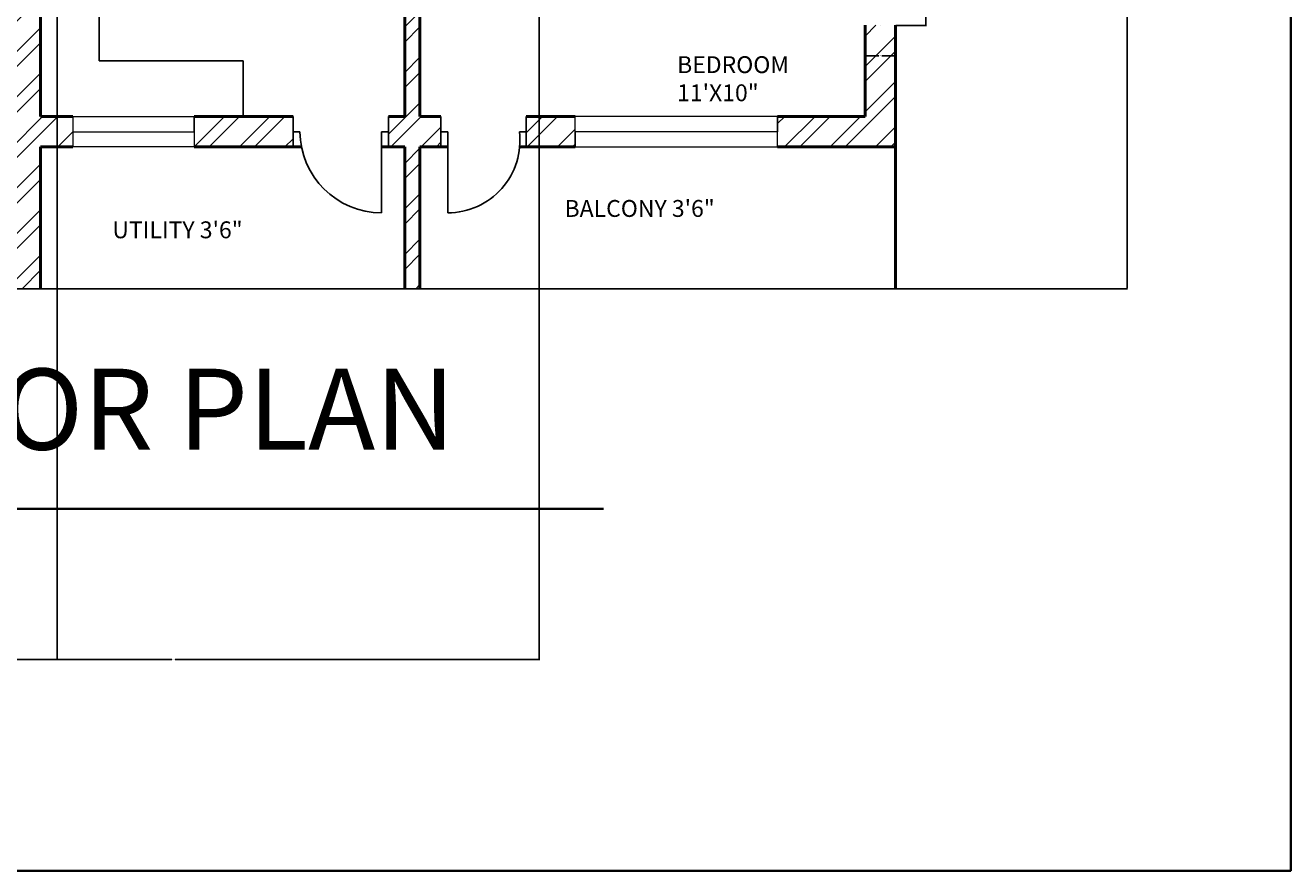
# Model space of a CAD drawing. Units: inches. Extents: x 1980 to 2738, y 1471 to 2568.
# Tile 11 of 22: x 2363 to 2738, y 1471 to 1722. Entities that reach past the tile are written whole.
import ezdxf

# ---------------------------------------------------------------- set-up
doc = ezdxf.new("R2010")
doc.units = ezdxf.units.IN
for name, color, linetype, lineweight in [('A-ANNO-DIMS', 2, 'Continuous', 18), ('A-ANNO-TTLB', 7, 'Continuous', 35), ('A-AREA-IDEN', 7, 'Continuous', 18), ('A-DOOR', 31, 'Continuous', 25), ('A-FLOR-BALC', 7, 'Continuous', 25), ('A-FLOR-CASE', 8, 'Continuous', 25), ('A-GLAZ', 141, 'Continuous', 18), ('A-WALL', 7, 'Continuous', 50)]:
    doc.layers.add(name, color=color, linetype=linetype, lineweight=lineweight)
doc.layers.add('A-WALL-PATT', color=9, linetype='Continuous', lineweight=13, true_color=0xd19cc7)
doc.styles.get("Standard").update_dxf_attribs({"font": 'arial.ttf'})
doc.dimstyles.get("Standard").update_dxf_attribs({"dimtxt": 0.18, "dimasz": 0.18, "dimexe": 0.18, "dimexo": 0.0625, "dimgap": 0.09, "dimtad": 0, "dimtih": 1, "dimtoh": 1, "dimdec": 4, "dimzin": 0, "dimdsep": 46, "dimtxsty": 'Standard', "dimcen": 0.09, "dimadec": 0, "dimazin": 0, "dimtfac": 1, "dimtdec": 4, "dimtofl": 0, "dimtmove": 0, "dimatfit": 3, "dimfxl": 1, "dimtolj": 1, "dimtzin": 0, "dimarcsym": 0})

# ---------------------------------------------------------------- blocks, each defined once
blk = doc.blocks.new('WIN-60IN-WALL')
for p, q in [((0, 9), (0, 0)), ((60, 9), (0, 9)), ((60, 4.5), (60, 9)), ((60, 9), (60, 0)), ((0, 0), (0, 4.5)), ((0, 4.5), (60, 4.5)), ((0, 0), (60, 0))]:
    blk.add_line(p, q)
blk = doc.blocks.new('*D29')
at = {"layer": 'A-ANNO-DIMS', "color": 0, "lineweight": -2, "transparency": 16777216}
for p, q in [((2621.15, 1781.73), (2630.26, 1781.73)), ((2630.08, 1781.55), (2630.08, 1751.92)), ((2630.08, 1721.91), (2630.08, 1751.55)), ((2621.15, 1721.73), (2630.26, 1721.73))]:
    blk.add_line(p, q, dxfattribs=at)
at = {"layer": 'A-ANNO-DIMS', "color": 0, "transparency": 16777216}
for points in [[(2630.05, 1781.55), (2630.11, 1781.55), (2630.08, 1781.73)], [(2630.05, 1721.91), (2630.11, 1721.91), (2630.08, 1721.73)]]:
    blk.add_solid(points, dxfattribs=at)
at = {"layer": 'Defpoints', "color": 0, "transparency": 16777216}
for p in [(2621.08, 1781.73), (2630.08, 1781.73), (2621.08, 1721.73)]:
    blk.add_point(p, dxfattribs=at)
at = {"layer": 'A-ANNO-DIMS', "color": 0, "transparency": 16777216, "insert": (2630.08, 1751.73), "char_height": 0.18, "attachment_point": 5}
blk.add_mtext('\\A1;WINDOW 60 TYP.', dxfattribs=at)
blk = doc.blocks.new('*D30')
at = {"layer": 'A-ANNO-DIMS', "color": 0, "lineweight": -2, "transparency": 16777216}
for p, q in [((2612.08, 1721.67), (2612.08, 1712.55)), ((2621.08, 1721.67), (2621.08, 1712.55)), ((2612.26, 1712.73), (2616.13, 1712.73)), ((2620.9, 1712.73), (2617.04, 1712.73))]:
    blk.add_line(p, q, dxfattribs=at)
at = {"layer": 'A-ANNO-DIMS', "color": 0, "transparency": 16777216}
for points in [[(2612.26, 1712.76), (2612.26, 1712.7), (2612.08, 1712.73)], [(2620.9, 1712.76), (2620.9, 1712.7), (2621.08, 1712.73)]]:
    blk.add_solid(points, dxfattribs=at)
at = {"layer": 'Defpoints', "color": 0, "transparency": 16777216}
for p in [(2612.08, 1721.73), (2621.08, 1721.73), (2621.08, 1712.73)]:
    blk.add_point(p, dxfattribs=at)
at = {"layer": 'A-ANNO-DIMS', "color": 0, "transparency": 16777216, "insert": (2616.58, 1712.73), "char_height": 0.18, "attachment_point": 5}
blk.add_mtext('\\A1;9 TYP.', dxfattribs=at)
blk = doc.blocks.new('*D37')
at = {"layer": 'A-ANNO-DIMS', "color": 0, "lineweight": -2, "transparency": 16777216}
for p, q in [((2579.97, 2011.21), (2689.91, 2011.21)), ((2689.73, 2011.03), (2689.73, 1827.64)), ((2689.73, 1643.89), (2689.73, 1827.27)), ((2621.15, 1643.71), (2689.91, 1643.71))]:
    blk.add_line(p, q, dxfattribs=at)
at = {"layer": 'A-ANNO-DIMS', "color": 0, "transparency": 16777216}
for points in [[(2689.7, 2011.03), (2689.76, 2011.03), (2689.73, 2011.21)], [(2689.7, 1643.89), (2689.76, 1643.89), (2689.73, 1643.71)]]:
    blk.add_solid(points, dxfattribs=at)
at = {"layer": 'Defpoints', "color": 0, "transparency": 16777216}
for p in [(2579.9, 2011.21), (2689.73, 2011.21), (2621.08, 1643.71)]:
    blk.add_point(p, dxfattribs=at)
at = {"layer": 'A-ANNO-DIMS', "color": 0, "transparency": 16777216, "insert": (2689.73, 1827.46), "char_height": 0.18, "attachment_point": 5}
blk.add_mtext('\\A1;367.5', dxfattribs=at)
blk = doc.blocks.new('*D41')
at = {"layer": 'A-ANNO-DIMS', "color": 0, "lineweight": -2, "transparency": 16777216}
for p, q in [((2298.65, 2095.14), (2298.65, 1533.71)), ((2515.4, 2095.14), (2515.4, 1533.71)), ((2298.83, 1533.89), (2406.56, 1533.89)), ((2515.22, 1533.89), (2407.49, 1533.89))]:
    blk.add_line(p, q, dxfattribs=at)
at = {"layer": 'A-ANNO-DIMS', "color": 0, "transparency": 16777216}
for points in [[(2298.83, 1533.92), (2298.83, 1533.86), (2298.65, 1533.89)], [(2515.22, 1533.92), (2515.22, 1533.86), (2515.4, 1533.89)]]:
    blk.add_solid(points, dxfattribs=at)
at = {"layer": 'Defpoints', "color": 0, "transparency": 16777216}
for p in [(2298.65, 2095.21), (2515.4, 2095.21), (2515.4, 1533.89)]:
    blk.add_point(p, dxfattribs=at)
at = {"layer": 'A-ANNO-DIMS', "color": 0, "transparency": 16777216, "insert": (2407.03, 1533.89), "char_height": 0.18, "attachment_point": 5}
blk.add_mtext('\\A1;216.75', dxfattribs=at)
blk = doc.blocks.new('*D57')
at = {"layer": 'A-ANNO-DIMS', "color": 0, "lineweight": -2, "transparency": 16777216}
for p, q in [((2351.81, 1792.14), (2351.81, 1533.71)), ((2372.53, 1792.14), (2372.53, 1533.71)), ((2351.99, 1533.89), (2361.77, 1533.89)), ((2372.35, 1533.89), (2362.56, 1533.89))]:
    blk.add_line(p, q, dxfattribs=at)
at = {"layer": 'A-ANNO-DIMS', "color": 0, "transparency": 16777216}
for points in [[(2351.99, 1533.92), (2351.99, 1533.86), (2351.81, 1533.89)], [(2372.35, 1533.92), (2372.35, 1533.86), (2372.53, 1533.89)]]:
    blk.add_solid(points, dxfattribs=at)
at = {"layer": 'Defpoints', "color": 0, "transparency": 16777216}
for p in [(2351.81, 1792.21), (2372.53, 1792.21), (2372.53, 1533.89)]:
    blk.add_point(p, dxfattribs=at)
at = {"layer": 'A-ANNO-DIMS', "color": 0, "transparency": 16777216, "insert": (2362.17, 1533.89), "char_height": 0.18, "attachment_point": 5}
blk.add_mtext('\\A1;20.72', dxfattribs=at)

msp = doc.modelspace()

# ---------------------------------------------------------------- hatches: boundary and pattern name
at = {"layer": 'A-WALL-PATT'}
h = msp.add_hatch(dxfattribs=at)
h.set_pattern_fill('ANSI32', color=256)
h.paths.add_polyline_path([(2257.5661, 2416.2064), (2257.5661, 2420.7064), (2250.5833, 2420.7064), (2250.5833, 2462.7064), (2246.0833, 2462.7064), (2246.0833, 2420.7064), (2237.0791, 2420.7064), (2237.0791, 2411.7064), (2246.0833, 2411.7064), (2246.0833, 2291.7064), (2242.6109, 2291.7064), (2242.6109, 2287.2064), (2246.0833, 2287.2064), (2250.5833, 2287.2064), (2250.5833, 2291.7064), (2250.5833, 2411.7064), (2257.5661, 2411.7064)])
h.paths.add_polyline_path([(2387.0396, 2416.2064), (2387.0396, 2420.7064), (2367.5833, 2420.7064), (2367.5833, 2462.7064), (2358.5833, 2462.7064), (2358.5833, 2420.7064), (2329.3087, 2420.7064), (2329.3087, 2411.7064), (2358.5833, 2411.7064), (2358.5833, 2321.7275), (2358.5833, 2309.7064), (2347.3089, 2309.7064), (2293.3089, 2309.7064), (2293.3089, 2259.0771), (2297.8089, 2259.0771), (2297.8089, 2305.2064), (2347.3089, 2305.2064), (2347.3089, 2284.7412), (2351.8089, 2284.7412), (2351.8089, 2305.2064), (2372.3188, 2305.2064), (2372.3761, 2284.3899), (2377.0295, 2284.3899), (2377.0295, 2299.3058), (2377.0295, 2305.2064), (2426.5295, 2305.2064), (2426.5295, 2257.5573), (2431.0295, 2257.5573), (2431.0295, 2309.7064), (2377.0295, 2309.7064), (2367.5833, 2309.7064), (2367.5833, 2321.7275), (2367.5833, 2411.7064), (2387.0396, 2411.7064)])
h.paths.add_polyline_path([(2448.5267, 2416.2064), (2448.5267, 2420.7064), (2423.0396, 2420.7064), (2423.0396, 2411.7064), (2448.5267, 2411.7064)])
h.paths.add_polyline_path([(2130.9128, 2416.2064), (2130.9128, 2420.7064), (2105.0833, 2420.7064), (2105.0833, 2386.6942), (2114.0833, 2386.6942), (2114.0833, 2411.7064), (2130.9128, 2411.7064)])
h.paths.add_polyline_path([(2212.9478, 2420.7064), (2190.9128, 2420.7064), (2190.9128, 2411.7064), (2212.9478, 2411.7064), (2212.9478, 2416.2064)])
h.paths.add_polyline_path([(2114.0833, 2326.6942), (2105.0833, 2326.6942), (2105.0833, 2291.7064), (2081.0833, 2291.7064), (2081.0833, 2287.2064), (2105.0833, 2287.2064), (2105.0833, 2276.1935), (2114.0833, 2276.1935), (2114.0833, 2287.2064), (2166.3825, 2287.2064), (2166.3825, 2289.4564), (2166.3825, 2291.7064), (2114.0833, 2291.7064)])
h.paths.add_polyline_path([(2114.0833, 2252.1935), (2105.0833, 2252.1935), (2105.0833, 2233.2064), (2081.0833, 2233.2064), (2081.0833, 2228.7064), (2105.0833, 2228.7064), (2105.0833, 2213.4478), (2114.0833, 2213.4478), (2114.0833, 2228.7064), (2195.0833, 2228.7064), (2199.5833, 2228.7064), (2208.4455, 2228.7064), (2208.4455, 2230.9564), (2208.4455, 2233.2064), (2199.5833, 2233.2064), (2199.5833, 2287.2064), (2206.8904, 2287.2064), (2206.8904, 2289.4564), (2206.8904, 2291.7064), (2189.446, 2291.7064), (2189.446, 2289.4564), (2189.446, 2287.2064), (2195.0833, 2287.2064), (2195.0833, 2233.2064), (2114.0833, 2233.2064)])
h.paths.add_polyline_path([(2114.0833, 2153.4478), (2109.5833, 2153.4478), (2105.0833, 2153.4478), (2105.0833, 2135.2374), (2114.0833, 2135.2374)], flags=17)
h.paths.add_polyline_path([(2135.9619, 2095.4081), (2140.1805, 2095.4081), (2140.1805, 2104.2064), (2114.0833, 2104.2064), (2114.0833, 2110.3997), (2109.5833, 2110.3997), (2105.0833, 2110.3997), (2105.0833, 2104.2064), (2081.0833, 2104.2064), (2081.0833, 2099.7064), (2105.0833, 2099.7064), (2127.5416, 2099.8532), (2127.5416, 2056.9393), (2136.2133, 2056.9393)], flags=17)
h.paths.add_polyline_path([(2255.4895, 2104.2064), (2250.5833, 2104.2064), (2250.5833, 2233.2064), (2246.0833, 2233.2064), (2242.4941, 2233.2064), (2242.4941, 2228.7064), (2246.0833, 2228.7064), (2246.0833, 2104.2064), (2163.6825, 2104.2064), (2163.6825, 2099.8072), (2163.6825, 2095.4081), (2191.4325, 2095.4081), (2191.4325, 2011.2064), (2186.0833, 2011.2064), (2136.5143, 2010.8824), (2136.3702, 2032.9403), (2131.9559, 2032.9115), (2127.5416, 2032.8826), (2127.5416, 2006.7064), (2105.0833, 2006.7064), (2081.0833, 2006.7064), (2081.0833, 2002.2064), (2105.0833, 2002.2064), (2105.0833, 1995.9329), (2114.0833, 1995.9329), (2114.0833, 2002.2064), (2246.0833, 2002.2064), (2246.0833, 1877.7064), (2242.1358, 1877.7064), (2242.1358, 1873.2064), (2250.5833, 1873.2064), (2250.5833, 2002.2064), (2255.3335, 2002.2064), (2255.3335, 2011.2064), (2195.9325, 2011.2064), (2195.9325, 2095.2064), (2255.4895, 2095.2064), (2255.4895, 2099.5471)])
h.paths.add_polyline_path([(2199.5833, 1873.2064), (2209.827, 1873.2064), (2209.827, 1875.4564), (2209.827, 1877.7064), (2114.0833, 1877.7064), (2114.0833, 1890.0968), (2105.0833, 1890.0968), (2105.0833, 1877.7064), (2081.0833, 1877.7064), (2081.0833, 1873.2064), (2105.0833, 1873.2064), (2105.0833, 1857.7279), (2114.0833, 1857.7279), (2114.0833, 1873.2064), (2195.0833, 1873.2064), (2195.0833, 1819.2064), (2190.298, 1819.2064), (2190.298, 1814.7064), (2209.8976, 1814.7064), (2209.8976, 1816.9564), (2209.8976, 1819.2064), (2199.5833, 1819.2064)])
h.paths.add_polyline_path([(2114.0833, 1814.7064), (2166.2538, 1814.7064), (2166.2538, 1816.9564), (2166.2538, 1819.2064), (2114.0833, 1819.2064), (2114.0833, 1833.7279), (2109.5833, 1833.7279), (2105.0833, 1833.7279), (2105.0833, 1819.2064), (2081.0833, 1819.2064), (2081.0833, 1814.7064), (2105.0833, 1814.7064), (2105.0833, 1782.5516), (2114.0833, 1782.5516)])
h.paths.add_polyline_path([(2114.0833, 1722.5516), (2109.5833, 1722.5516), (2105.0833, 1722.5516), (2105.0833, 1685.7064), (2124.5104, 1685.7064), (2124.5104, 1690.2064), (2124.5104, 1694.7064), (2114.0833, 1694.7064)])
h.paths.add_polyline_path([(2218.8787, 1694.7064), (2184.5104, 1694.7064), (2184.5104, 1685.7064), (2218.8787, 1685.7064), (2218.8787, 1690.2064)])
h.paths.add_polyline_path([(2250.5833, 1819.2064), (2242.6431, 1819.2064), (2242.6431, 1816.9564), (2242.6431, 1814.7064), (2246.0833, 1814.7064), (2246.0833, 1694.7064), (2240.4035, 1694.7064), (2240.4035, 1690.2064), (2240.4035, 1685.7064), (2246.0833, 1685.7064), (2246.0833, 1643.7064), (2250.5833, 1643.7064), (2250.5833, 1685.7064), (2255.9859, 1685.7064), (2255.9859, 1690.2064), (2255.9859, 1694.7064), (2250.5833, 1694.7064)])
h.paths.add_polyline_path([(2297.4764, 1694.7064), (2279.3934, 1694.7064), (2279.3934, 1690.2064), (2279.3934, 1685.7064), (2297.4764, 1685.7064), (2297.4764, 1690.2064)])
h.paths.add_polyline_path([(2377.1596, 1694.7064), (2367.5833, 1694.7064), (2367.5833, 1787.7064), (2431.0295, 1787.7064), (2431.0295, 1792.2064), (2431.0295, 1849.4149), (2428.7795, 1849.4149), (2426.5295, 1849.4149), (2426.5295, 1792.2064), (2421.5833, 1792.2064), (2367.5833, 1792.2064), (2297.8089, 1792.2064), (2297.8089, 1850.2946), (2295.5589, 1850.2946), (2293.3089, 1850.2946), (2293.3089, 1792.2064), (2293.3089, 1787.7064), (2297.8089, 1787.7064), (2358.5833, 1787.7064), (2358.5833, 1694.7064), (2333.4764, 1694.7064), (2333.4764, 1685.7064), (2358.5833, 1685.7064), (2358.5833, 1643.7064), (2367.5833, 1643.7064), (2367.5833, 1685.7064), (2377.1596, 1685.7064)])
h.paths.add_polyline_path([(2442.4912, 1694.7064), (2413.1596, 1694.7064), (2413.1596, 1685.7064), (2442.4912, 1685.7064)])
h.paths.add_polyline_path([(2480.0833, 1814.7064), (2483.4816, 1814.7064), (2483.4816, 1817.9384), (2483.4816, 1819.2064), (2475.5833, 1819.2064), (2475.5833, 1694.7064), (2470.7283, 1694.7064), (2470.7283, 1685.7064), (2475.5833, 1685.7064), (2475.5833, 1643.7064), (2480.0833, 1643.7064), (2480.0833, 1685.7064), (2486.3293, 1685.7064), (2486.3293, 1690.2064), (2486.3293, 1694.7064), (2480.0833, 1694.7064)])
h.paths.add_polyline_path([(2621.0833, 1721.7349), (2612.0833, 1721.7349), (2612.0833, 1694.7064), (2586.1453, 1694.7064), (2586.1453, 1685.7064), (2621.0833, 1685.7064)])
h.paths.add_polyline_path([(2526.1453, 1690.2064), (2526.1453, 1694.7064), (2511.584, 1694.7064), (2511.584, 1690.2064), (2511.584, 1685.7064), (2526.1453, 1685.7064)])
h.paths.add_polyline_path([(2645.0833, 1819.2064), (2621.0833, 1819.2064), (2621.0833, 1835.8527), (2616.5833, 1835.8527), (2612.0833, 1835.8527), (2612.0833, 1819.2064), (2560.2541, 1819.2064), (2560.2541, 1814.7064), (2612.0833, 1814.7064), (2612.0833, 1781.7349), (2621.0833, 1781.7349), (2621.0833, 1814.7064), (2645.0833, 1814.7064)])
h.paths.add_polyline_path([(2645.0833, 1877.7064), (2621.0833, 1877.7064), (2621.0833, 1886.4375), (2612.0833, 1886.4375), (2612.0833, 1877.7064), (2517.1032, 1877.7064), (2517.1032, 1875.4564), (2517.1032, 1873.2064), (2526.5833, 1873.2064), (2526.5833, 1819.2064), (2516.6454, 1819.2064), (2516.6454, 1816.9564), (2516.6454, 1814.7064), (2536.4445, 1814.7064), (2536.4445, 1816.9564), (2536.4445, 1819.2064), (2531.0833, 1819.2064), (2531.0833, 1873.2064), (2612.0833, 1873.2064), (2612.0833, 1859.8527), (2621.0833, 1859.8527), (2621.0833, 1873.2064), (2645.0833, 1873.2064)])
h.paths.add_polyline_path([(2645.0833, 2006.7064), (2621.0833, 2006.7064), (2588.5085, 2006.7064), (2588.5085, 2052.9125), (2579.9045, 2052.9125), (2579.9045, 2011.2064), (2519.9045, 2011.2064), (2519.9045, 2095.2064), (2553.1204, 2095.2064), (2553.1204, 2104.2064), (2480.0833, 2104.2064), (2480.0833, 2228.7064), (2484.3832, 2228.7064), (2484.3832, 2230.9564), (2484.3832, 2233.2064), (2475.5833, 2233.2064), (2475.5833, 2104.2064), (2463.1308, 2104.2064), (2463.1308, 2095.2064), (2501.2463, 2095.2064), (2510.9045, 2095.2064), (2515.4045, 2095.2064), (2515.4045, 2011.2064), (2510.9045, 2011.2064), (2501.2463, 2011.2064), (2462.5957, 2011.2064), (2462.5957, 2002.2064), (2475.5833, 2002.2064), (2475.5833, 1873.2064), (2483.6146, 1873.2064), (2483.6146, 1875.4564), (2483.6146, 1877.7064), (2480.0833, 1877.7064), (2480.0833, 2002.2064), (2612.0833, 2002.2064), (2612.0833, 1996.309), (2621.0833, 1996.309), (2621.0833, 2002.2064), (2645.0833, 2002.2064)])
h.paths.add_polyline_path([(2588.5085, 2099.7277), (2621.0833, 2099.7277), (2645.0833, 2099.7064), (2645.0833, 2104.2064), (2621.0833, 2104.2064), (2621.0833, 2109.0038), (2616.5833, 2109.0038), (2612.0833, 2109.0038), (2612.0833, 2104.2064), (2575.0621, 2104.2064), (2575.0621, 2099.7064), (2575.0621, 2095.2064), (2579.9045, 2095.2064), (2579.9045, 2076.9125), (2588.5085, 2076.9125)], flags=17)
h.paths.add_polyline_path([(2367.5833, 2002.2064), (2373.7228, 2002.2064), (2373.7228, 2006.7064), (2373.7228, 2011.2064), (2350.7889, 2011.2064), (2350.7889, 2006.7064), (2350.7889, 2002.2064), (2358.5833, 2002.2064), (2358.5833, 1877.7064), (2293.3089, 1877.7064), (2293.3089, 1870.4987), (2297.8089, 1870.4987), (2297.8089, 1873.2064), (2347.3089, 1873.2064), (2347.3089, 1847.2208), (2351.8089, 1847.2208), (2351.8089, 1873.2064), (2372.5295, 1873.2064), (2372.5295, 1847.8619), (2377.0295, 1847.8619), (2377.0295, 1873.2064), (2426.5295, 1873.2064), (2426.5295, 1868.7339), (2431.0295, 1868.7339), (2431.0295, 1877.7064), (2367.5833, 1877.7064)])
h.paths.add_polyline_path([(2531.0833, 2287.2064), (2534.2285, 2287.2064), (2534.2285, 2291.7064), (2516.7886, 2291.7064), (2516.7886, 2287.2064), (2526.5833, 2287.2064), (2526.5833, 2233.2064), (2517.9112, 2233.2064), (2517.9112, 2230.9564), (2517.9112, 2228.7064), (2526.5833, 2228.7064), (2531.0833, 2228.7064), (2612.0833, 2228.7064), (2612.0833, 2206.8504), (2621.0833, 2206.8504), (2621.0833, 2228.7064), (2645.0833, 2228.7064), (2645.0833, 2233.2064), (2621.0833, 2233.2064), (2621.0833, 2241.8536), (2616.5833, 2241.8536), (2612.0833, 2241.8536), (2612.0833, 2233.2064), (2531.0833, 2233.2064)])
h.paths.add_polyline_path([(2645.0833, 2291.7064), (2621.0833, 2291.7064), (2621.0833, 2323.0138), (2616.5833, 2323.0138), (2612.0833, 2323.0138), (2612.0833, 2291.7064), (2559.6852, 2291.7064), (2559.6852, 2289.4564), (2559.6852, 2287.2064), (2612.0833, 2287.2064), (2612.0833, 2265.8536), (2621.0833, 2265.8536), (2621.0833, 2287.2064), (2645.0833, 2287.2064)])
h.paths.add_polyline_path([(2621.0833, 2420.7064), (2582.8189, 2420.7064), (2582.8189, 2411.7064), (2612.0833, 2411.7064), (2612.0833, 2383.0138), (2621.0833, 2383.0138)])
h.paths.add_polyline_path([(2480.0833, 2411.7064), (2485.7342, 2411.7064), (2485.7342, 2416.2064), (2485.7342, 2420.7064), (2480.0833, 2420.7064), (2480.0833, 2462.7064), (2475.5833, 2462.7064), (2475.5833, 2420.7064), (2469.4083, 2420.7064), (2469.4083, 2411.7064), (2475.5833, 2411.7064), (2475.5833, 2291.7064), (2475.5833, 2287.2064), (2482.9195, 2287.2064), (2482.9195, 2289.4564), (2482.9195, 2291.7064), (2480.0833, 2291.7064)])
h.paths.add_polyline_path([(2367.5833, 2228.7064), (2431.0295, 2228.7064), (2431.0295, 2233.2064), (2431.0295, 2237.4203), (2428.7795, 2237.4203), (2426.5295, 2237.4203), (2426.5295, 2233.2064), (2377.0295, 2233.2064), (2377.0295, 2260.3837), (2372.4423, 2260.3837), (2372.517, 2233.2635), (2351.8089, 2233.2064), (2351.8089, 2260.7412), (2347.3089, 2260.7412), (2347.3089, 2233.2064), (2297.8089, 2233.2064), (2297.8089, 2236.9324), (2293.3089, 2236.9324), (2293.3089, 2228.7064), (2358.5833, 2228.7064), (2358.5833, 2104.2064), (2353.3665, 2104.2064), (2353.3665, 2095.2064), (2373.8869, 2095.2064), (2373.8869, 2099.7064), (2373.8869, 2104.2064), (2367.5833, 2104.2064)])
h.paths.add_polyline_path([(2321.2323, 2104.2064), (2303.4895, 2104.2064), (2303.4895, 2095.2064), (2321.2323, 2095.2064), (2321.2323, 2099.7064)], flags=0)
h.paths.add_polyline_path([(2415.1308, 2099.7064), (2415.1308, 2104.2064), (2404.81, 2104.2064), (2404.81, 2095.2064), (2415.1308, 2095.2064)], flags=17)
h.paths.add_polyline_path([(2318.6336, 2011.2064), (2303.3335, 2011.2064), (2303.3335, 2002.2064), (2318.6336, 2002.2064)], flags=0)
h.paths.add_polyline_path([(2414.5957, 2011.2064), (2406.2461, 2011.2064), (2406.2461, 2006.7064), (2406.2461, 2002.2064), (2414.5957, 2002.2064)], flags=17)

# ---------------------------------------------------------------- linework, layer by layer
at = {"layer": 'A-ANNO-TTLB'}
msp.add_line((2167.6271, 1578.5357), (2534.552, 1578.5357), dxfattribs=at)
msp.add_lwpolyline([(1979.5621, 2567.5568), (2738.2543, 2567.5568), (2738.2543, 1471.317), (1979.5621, 1471.317)], close=True, dxfattribs=at)
at = {"layer": 'A-DOOR'}
for p, q in [((2442.4912, 1685.7064), (2442.4912, 1694.7064)), ((2442.4912, 1694.7064), (2442.4912, 1690.2064)), ((2470.7283, 1694.7064), (2470.7283, 1685.7064)), ((2486.3293, 1694.7064), (2486.3293, 1685.7064)), ((2511.584, 1685.7064), (2511.584, 1694.7064)), ((2511.584, 1694.7064), (2511.584, 1690.2064)), ((2442.4912, 1690.2064), (2444.4912, 1690.2064)), ((2470.7283, 1690.2064), (2468.7283, 1690.2064)), ((2468.7283, 1690.2064), (2468.7283, 1666.2064)), ((2470.7283, 1685.7064), (2470.7283, 1690.2064)), ((2486.3293, 1685.7064), (2486.3293, 1690.2064)), ((2486.3293, 1690.2064), (2488.3293, 1690.2064)), ((2488.3293, 1690.2064), (2488.3293, 1666.2064)), ((2511.584, 1690.2064), (2509.584, 1690.2064))]:
    msp.add_line(p, q, dxfattribs=at)
for centre, radius, start, end in [((2468.7283, 1690.4448), 24.2383, 180.563418, 270), ((2488.3293, 1687.6182), 21.4118, 270, 6.942841)]:
    msp.add_arc(centre, radius, start, end, dxfattribs=at)
at = {"layer": 'A-FLOR-BALC'}
msp.add_line((2621.0833, 1643.7064), (2105.0833, 1643.7064), dxfattribs=at)
at = {"layer": 'A-FLOR-CASE'}
for p, q in [((2384.9917, 1787.7064), (2384.9917, 1711.1804)), ((2384.9917, 1711.1804), (2427.6819, 1711.1804)), ((2427.6819, 1711.1804), (2427.6819, 1694.7064))]:
    msp.add_line(p, q, dxfattribs=at)
at = {"layer": 'A-GLAZ'}
for p, q in [((2616.5833, 1721.7349), (2616.5833, 1721.7349)), ((2377.1596, 1694.7064), (2377.1596, 1685.7064)), ((2377.1596, 1694.7064), (2413.1596, 1694.7064)), ((2413.1596, 1690.2064), (2413.1596, 1694.7064)), ((2413.1596, 1694.7064), (2413.1596, 1694.7064)), ((2413.1596, 1694.7064), (2413.1596, 1685.7064)), ((2377.1596, 1690.2064), (2413.1596, 1690.2064)), ((2377.1596, 1685.7064), (2377.1596, 1685.7064)), ((2413.1596, 1685.7064), (2377.1596, 1685.7064))]:
    msp.add_line(p, q, dxfattribs=at)
at = {"layer": 'A-WALL'}
for p, q in [((2475.5833, 1819.2064), (2475.5833, 1694.7064)), ((2480.0833, 1814.7064), (2480.0833, 1694.7064)), ((2367.5833, 1787.7064), (2367.5833, 1694.7064)), ((2612.0833, 1721.7349), (2612.0833, 1694.7064)), ((2621.0833, 1721.7349), (2621.0833, 1643.7064)), ((2377.1596, 1694.7064), (2367.5833, 1694.7064)), ((2442.4912, 1694.7064), (2413.1596, 1694.7064)), ((2475.5833, 1694.7064), (2470.7283, 1694.7064)), ((2486.3293, 1694.7064), (2480.0833, 1694.7064)), ((2526.1453, 1694.7064), (2511.584, 1694.7064)), ((2612.0833, 1694.7064), (2586.1453, 1694.7064)), ((2367.5833, 1685.7064), (2367.5833, 1643.7064)), ((2377.1596, 1685.7064), (2367.5833, 1685.7064)), ((2444.9577, 1685.7064), (2413.1596, 1685.7064)), ((2475.5833, 1685.7064), (2468.7283, 1685.7064)), ((2475.5833, 1685.7064), (2475.5833, 1643.7064)), ((2480.0833, 1685.7064), (2480.0833, 1643.7064)), ((2488.3293, 1685.7064), (2480.0833, 1685.7064)), ((2526.1453, 1685.7064), (2509.6555, 1685.7064)), ((2621.0833, 1685.7064), (2586.1453, 1685.7064))]:
    msp.add_line(p, q, dxfattribs=at)

# ---------------------------------------------------------------- block references
at = {"layer": 'A-GLAZ', "rotation": 180}
msp.add_blockref('WIN-60IN-WALL', (2586.1451, 1694.7068), dxfattribs=at)

# ---------------------------------------------------------------- texts
at = {"layer": 'A-ANNO-TTLB', "insert": (2200.9148, 1620.0295), "char_height": 24, "attachment_point": 1}
msp.add_mtext_dynamic_manual_height_columns('FIRST FLOOR PLAN', width=445.461587, gutter_width=12.5, heights=[0], dxfattribs=at)
at = {"layer": 'A-AREA-IDEN', "char_height": 5, "attachment_point": 1}
for s, width, insert in [('BEDROOM\\P11\'X10"', 118.949412, (2556.3329, 1712.5843)), ('BALCONY 3\'6"', 63.132838, (2522.9546, 1669.9873)), ('UTILITY 3\'6"', 160.682584, (2388.8765, 1663.6555))]:
    msp.add_mtext_dynamic_manual_height_columns(s, width=width, gutter_width=12.5, heights=[0], dxfattribs=dict(at, insert=insert))

# ---------------------------------------------------------------- dimensions: what is measured, and where the dimension line sits
at = {"layer": 'A-ANNO-DIMS'}
for base, p1, p2, picture, middle in [((2515.4045, 1533.8857), (2298.6516, 2095.2064), (2515.4045, 2095.2064), '*D41', (2407.0281, 1533.8857)), ((2372.5295, 1533.8857), (2351.8089, 1792.2064), (2372.5295, 1792.2064), '*D57', (2362.1692, 1533.8857))]:
    dim = msp.add_linear_dim(base=base, p1=p1, p2=p2, dimstyle='Standard', override={"dimdec": 2, "dimlfac": 1, "dimrnd": 0, "dimzin": 0, "dimdsep": 46, "dimlunit": 2}, dxfattribs=at)
    dim.commit()
    dim.dimension.update_dxf_attribs({"geometry": picture, "text_midpoint": middle})
dim = msp.add_linear_dim(base=(2689.7333, 2011.2064), p1=(2621.0833, 1643.7064), p2=(2579.9045, 2011.2064), angle=90, dimstyle='Standard', override={"dimdec": 1, "dimlfac": 1, "dimrnd": 0, "dimzin": 0, "dimdsep": 46, "dimlunit": 2}, dxfattribs=at)
dim.commit()
dim.dimension.update_dxf_attribs({"geometry": '*D37', "text_midpoint": (2689.7333, 1827.4564)})
dim = msp.add_linear_dim(base=(2630.0833, 1781.7349), p1=(2621.0833, 1721.7349), p2=(2621.0833, 1781.7349), angle=90, text='WINDOW <> TYP.', dimstyle='Standard', override={"dimdec": 0, "dimlfac": 1, "dimrnd": 0, "dimzin": 0, "dimdsep": 46, "dimlunit": 2}, dxfattribs=at)
dim.commit()
dim.dimension.update_dxf_attribs({"geometry": '*D29', "text_midpoint": (2630.0833, 1751.7349)})
dim = msp.add_linear_dim(base=(2621.0833, 1712.7349), p1=(2612.0833, 1721.7349), p2=(2621.0833, 1721.7349), text='<> TYP.', dimstyle='Standard', override={"dimdec": 0, "dimlfac": 1, "dimrnd": 0, "dimzin": 0, "dimdsep": 46, "dimlunit": 2}, dxfattribs=at)
dim.commit()
dim.dimension.update_dxf_attribs({"geometry": '*D30', "text_midpoint": (2616.5833, 1712.7349)})

doc.saveas('drawing.dxf')
